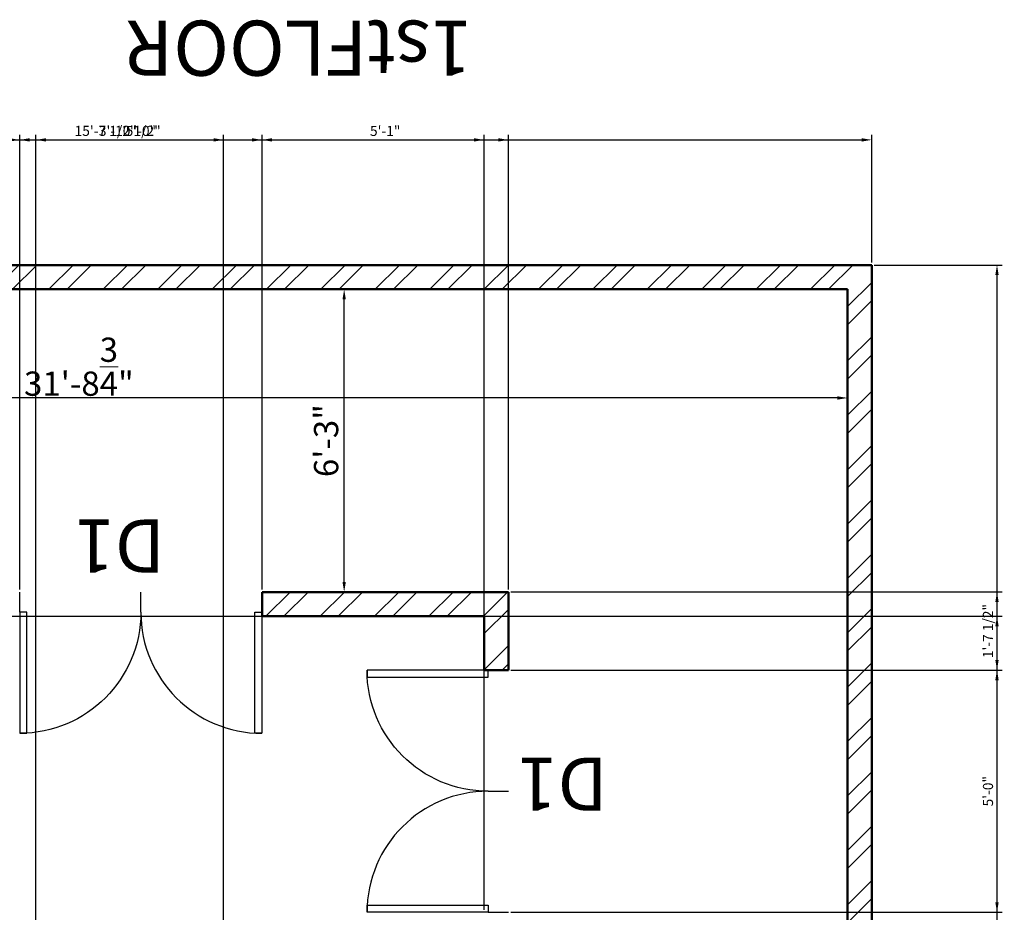
# Model space of a CAD drawing. Units: inches. Extents: x 244 to 2800, y 1060 to 1700.
# Tile 11 of 13: x 1781 to 2025, y 1473 to 1694. Entities that reach past the tile are written whole.
import ezdxf

# ---------------------------------------------------------------- set-up
doc = ezdxf.new("R2010")
doc.units = ezdxf.units.IN
for name, color, linetype, lineweight in [('A-ANNO-DIMS', 2, 'Continuous', 18), ('A-ANNO-TEXT', 1, 'Continuous', 18), ('A-DOOR', 5, 'Continuous', 25), ('A-WALL', 7, 'Continuous', 50), ('A-WALL-PATT', 8, 'Continuous', 13)]:
    doc.layers.add(name, color=color, linetype=linetype, lineweight=lineweight)
doc.styles.get("Standard").update_dxf_attribs({"font": 'arial.ttf'})
doc.dimstyles.new('ISO-25', dxfattribs={"dimtxt": 2.5, "dimasz": 2.5, "dimexe": 1.25, "dimexo": 0.625, "dimtad": 1, "dimlunit": 4, "dimtxsty": 'Standard', "dimcen": 2.5, "dimadec": 0, "dimazin": 0, "dimtfac": 1, "dimtmove": 0, "dimatfit": 3, "dimfxl": 1, "dimarcsym": 0})

# ---------------------------------------------------------------- blocks, each defined once
blk = doc.blocks.new('*U2')
for p, q in [((0, 0), (0, -5)), ((30, 0), (30, -5))]:
    blk.add_line(p, q)
blk.add_lwpolyline([(0, 0), (0, 30), (1.75, 30), (1.75, 0)], close=True)
blk.add_arc((0, 0), 30, 0, 90)
blk = doc.blocks.new('*D28')
at = {"layer": 'A-ANNO-DIMS', "color": 0, "lineweight": -2, "transparency": 16777216}
for p, q in [((1871.27, 1626.99), (1860.49, 1626.99)), ((1861.74, 1554.49), (1861.74, 1624.49)), ((1871.27, 1551.99), (1860.49, 1551.99))]:
    blk.add_line(p, q, dxfattribs=at)
at = {"layer": 'A-ANNO-DIMS', "color": 0, "transparency": 16777216}
for points in [[(1861.33, 1624.49), (1862.16, 1624.49), (1861.74, 1626.99)], [(1861.33, 1554.49), (1862.16, 1554.49), (1861.74, 1551.99)]]:
    blk.add_solid(points, dxfattribs=at)
at = {"layer": 'Defpoints', "color": 0, "transparency": 16777216}
for p in [(1861.74, 1626.99), (1871.9, 1626.99), (1871.9, 1551.99)]:
    blk.add_point(p, dxfattribs=at)
at = {"layer": 'A-ANNO-DIMS', "color": 0, "transparency": 16777216, "insert": (1858.05, 1589.49), "char_height": 6, "attachment_point": 5, "rotation": 90}
blk.add_mtext('6\'-3"', dxfattribs=at)
blk = doc.blocks.new('*D29')
at = {"layer": 'A-ANNO-DIMS', "color": 0, "lineweight": -2, "transparency": 16777216}
for p, q in [((1605.7, 1600.68), (1605.7, 1601.31)), ((1983.9, 1600.06), (1608.2, 1600.06)), ((1986.4, 1600.68), (1986.4, 1601.31))]:
    blk.add_line(p, q, dxfattribs=at)
at = {"layer": 'A-ANNO-DIMS', "color": 0, "transparency": 16777216}
for points in [[(1608.2, 1600.47), (1608.2, 1599.64), (1605.7, 1600.06)], [(1983.9, 1600.47), (1983.9, 1599.64), (1986.4, 1600.06)]]:
    blk.add_solid(points, dxfattribs=at)
at = {"layer": 'Defpoints', "color": 0, "transparency": 16777216}
for p in [(1605.7, 1600.06), (1605.7, 1600.06), (1986.4, 1600.06)]:
    blk.add_point(p, dxfattribs=at)
at = {"layer": 'A-ANNO-DIMS', "color": 0, "transparency": 16777216, "insert": (1796.05, 1607.8), "char_height": 6, "attachment_point": 5}
blk.add_mtext('31\'-8{\\H1x;\\S3/4;}"', dxfattribs=at)
blk = doc.blocks.new('*D74')
at = {"layer": 'A-ANNO-DIMS', "color": 0, "lineweight": -2, "transparency": 16777216}
for p, q in [((1512.4, 1633.61), (1512.4, 1665.24)), ((1992.4, 1633.61), (1992.4, 1665.24)), ((1514.9, 1663.99), (1989.9, 1663.99))]:
    blk.add_line(p, q, dxfattribs=at)
at = {"layer": 'A-ANNO-DIMS', "color": 0, "transparency": 16777216}
for points in [[(1514.9, 1664.4), (1514.9, 1663.57), (1512.4, 1663.99)], [(1989.9, 1664.4), (1989.9, 1663.57), (1992.4, 1663.99)]]:
    blk.add_solid(points, dxfattribs=at)
at = {"layer": 'Defpoints', "color": 0, "transparency": 16777216}
for p in [(1992.4, 1663.99), (1512.4, 1632.99), (1992.4, 1632.99)]:
    blk.add_point(p, dxfattribs=at)
at = {"layer": 'A-ANNO-DIMS', "color": 0, "transparency": 16777216, "insert": (1752.4, 1665.89), "char_height": 2.5, "attachment_point": 5}
blk.add_mtext('40\'-0"', dxfattribs=at)
blk = doc.blocks.new('*D75')
at = {"layer": 'A-ANNO-DIMS', "color": 0, "lineweight": -2, "transparency": 16777216}
for p, q in [((1993.02, 1632.99), (2024.65, 1632.99)), ((2023.4, 1095.49), (2023.4, 1630.49)), ((1993.02, 1092.99), (2024.65, 1092.99))]:
    blk.add_line(p, q, dxfattribs=at)
at = {"layer": 'A-ANNO-DIMS', "color": 0, "transparency": 16777216}
for points in [[(2022.98, 1630.49), (2023.81, 1630.49), (2023.4, 1632.99)], [(2022.98, 1095.49), (2023.81, 1095.49), (2023.4, 1092.99)]]:
    blk.add_solid(points, dxfattribs=at)
at = {"layer": 'Defpoints', "color": 0, "transparency": 16777216}
for p in [(1992.4, 1632.99), (2023.4, 1632.99), (1992.4, 1092.99)]:
    blk.add_point(p, dxfattribs=at)
at = {"layer": 'A-ANNO-DIMS', "color": 0, "transparency": 16777216, "insert": (2021.49, 1362.99), "char_height": 2.5, "attachment_point": 5, "rotation": 90}
blk.add_mtext('45\'-0"', dxfattribs=at)
blk = doc.blocks.new('*D78')
at = {"layer": 'A-ANNO-DIMS', "color": 0, "lineweight": -2, "transparency": 16777216}
for p, q in [((1756.81, 1552.61), (1756.81, 1665.24)), ((1781.4, 1552.61), (1781.4, 1665.24)), ((1759.31, 1663.99), (1778.9, 1663.99))]:
    blk.add_line(p, q, dxfattribs=at)
at = {"layer": 'A-ANNO-DIMS', "color": 0, "transparency": 16777216}
for points in [[(1759.31, 1664.4), (1759.31, 1663.57), (1756.81, 1663.99)], [(1778.9, 1664.4), (1778.9, 1663.57), (1781.4, 1663.99)]]:
    blk.add_solid(points, dxfattribs=at)
at = {"layer": 'Defpoints', "color": 0, "transparency": 16777216}
for p in [(1781.4, 1663.99), (1756.81, 1551.99), (1781.4, 1551.99)]:
    blk.add_point(p, dxfattribs=at)
at = {"layer": 'A-ANNO-DIMS', "color": 0, "transparency": 16777216, "insert": (1769.1, 1665.9), "char_height": 2.5, "attachment_point": 5}
blk.add_mtext('2\'-0 1/2"', dxfattribs=at)
blk = doc.blocks.new('*D79')
at = {"layer": 'A-ANNO-DIMS', "color": 0, "lineweight": -2, "transparency": 16777216}
for p, q in [((1781.4, 1552.61), (1781.4, 1665.24)), ((1841.4, 1552.61), (1841.4, 1665.24)), ((1783.9, 1663.99), (1838.9, 1663.99))]:
    blk.add_line(p, q, dxfattribs=at)
at = {"layer": 'A-ANNO-DIMS', "color": 0, "transparency": 16777216}
for points in [[(1783.9, 1664.4), (1783.9, 1663.57), (1781.4, 1663.99)], [(1838.9, 1664.4), (1838.9, 1663.57), (1841.4, 1663.99)]]:
    blk.add_solid(points, dxfattribs=at)
at = {"layer": 'Defpoints', "color": 0, "transparency": 16777216}
for p in [(1841.4, 1663.99), (1781.4, 1551.99), (1841.4, 1551.99)]:
    blk.add_point(p, dxfattribs=at)
at = {"layer": 'A-ANNO-DIMS', "color": 0, "transparency": 16777216, "insert": (1811.4, 1665.89), "char_height": 2.5, "attachment_point": 5}
blk.add_mtext('5\'-0"', dxfattribs=at)
blk = doc.blocks.new('*D80')
at = {"layer": 'A-ANNO-DIMS', "color": 0, "lineweight": -2, "transparency": 16777216}
for p, q in [((1841.4, 1552.61), (1841.4, 1665.24)), ((1902.4, 1552.61), (1902.4, 1665.24)), ((1843.9, 1663.99), (1899.9, 1663.99))]:
    blk.add_line(p, q, dxfattribs=at)
at = {"layer": 'A-ANNO-DIMS', "color": 0, "transparency": 16777216}
for points in [[(1843.9, 1664.4), (1843.9, 1663.57), (1841.4, 1663.99)], [(1899.9, 1664.4), (1899.9, 1663.57), (1902.4, 1663.99)]]:
    blk.add_solid(points, dxfattribs=at)
at = {"layer": 'Defpoints', "color": 0, "transparency": 16777216}
for p in [(1902.4, 1663.99), (1841.4, 1551.99), (1902.4, 1551.99)]:
    blk.add_point(p, dxfattribs=at)
at = {"layer": 'A-ANNO-DIMS', "color": 0, "transparency": 16777216, "insert": (1871.9, 1665.89), "char_height": 2.5, "attachment_point": 5}
blk.add_mtext('5\'-1"', dxfattribs=at)
blk = doc.blocks.new('*D87')
at = {"layer": 'A-ANNO-DIMS', "color": 0, "lineweight": -2, "transparency": 16777216}
for p, q in [((1537.02, 1545.99), (2024.65, 1545.99)), ((2023.4, 1375.49), (2023.4, 1543.49)), ((1537.02, 1372.99), (2024.65, 1372.99))]:
    blk.add_line(p, q, dxfattribs=at)
at = {"layer": 'A-ANNO-DIMS', "color": 0, "transparency": 16777216}
for points in [[(2022.98, 1543.49), (2023.81, 1543.49), (2023.4, 1545.99)], [(2022.98, 1375.49), (2023.81, 1375.49), (2023.4, 1372.99)]]:
    blk.add_solid(points, dxfattribs=at)
at = {"layer": 'Defpoints', "color": 0, "transparency": 16777216}
for p in [(1536.4, 1545.99), (2023.4, 1545.99), (1536.4, 1372.99)]:
    blk.add_point(p, dxfattribs=at)
at = {"layer": 'A-ANNO-DIMS', "color": 0, "transparency": 16777216, "insert": (2021.49, 1459.49), "char_height": 2.5, "attachment_point": 5, "rotation": 90}
blk.add_mtext('14\'-5"', dxfattribs=at)
blk = doc.blocks.new('*D90')
at = {"layer": 'A-ANNO-DIMS', "color": 0, "lineweight": -2, "transparency": 16777216}
for p, q in [((1708.9, 1491.26), (1708.9, 1665.24)), ((1896.4, 1473.26), (1896.4, 1665.24)), ((1711.4, 1663.99), (1893.9, 1663.99))]:
    blk.add_line(p, q, dxfattribs=at)
at = {"layer": 'A-ANNO-DIMS', "color": 0, "transparency": 16777216}
for points in [[(1711.4, 1664.4), (1711.4, 1663.57), (1708.9, 1663.99)], [(1893.9, 1664.4), (1893.9, 1663.57), (1896.4, 1663.99)]]:
    blk.add_solid(points, dxfattribs=at)
at = {"layer": 'Defpoints', "color": 0, "transparency": 16777216}
for p in [(1896.4, 1663.99), (1708.9, 1490.64), (1896.4, 1472.64)]:
    blk.add_point(p, dxfattribs=at)
at = {"layer": 'A-ANNO-DIMS', "color": 0, "transparency": 16777216, "insert": (1802.65, 1665.9), "char_height": 2.5, "attachment_point": 5}
blk.add_mtext('15\'-7 1/2"', dxfattribs=at)
blk = doc.blocks.new('*D100')
at = {"layer": 'A-ANNO-DIMS', "color": 0, "lineweight": -2, "transparency": 16777216}
for p, q in [((1903.02, 1532.64), (2024.65, 1532.64)), ((2023.4, 1475.14), (2023.4, 1530.14)), ((1903.02, 1472.64), (2024.65, 1472.64))]:
    blk.add_line(p, q, dxfattribs=at)
at = {"layer": 'A-ANNO-DIMS', "color": 0, "transparency": 16777216}
for points in [[(2022.98, 1530.14), (2023.81, 1530.14), (2023.4, 1532.64)], [(2022.98, 1475.14), (2023.81, 1475.14), (2023.4, 1472.64)]]:
    blk.add_solid(points, dxfattribs=at)
at = {"layer": 'Defpoints', "color": 0, "transparency": 16777216}
for p in [(1902.4, 1532.64), (2023.4, 1532.64), (1902.4, 1472.64)]:
    blk.add_point(p, dxfattribs=at)
at = {"layer": 'A-ANNO-DIMS', "color": 0, "transparency": 16777216, "insert": (2021.49, 1502.64), "char_height": 2.5, "attachment_point": 5, "rotation": 90}
blk.add_mtext('5\'-0"', dxfattribs=at)
blk = doc.blocks.new('*D101')
at = {"layer": 'A-ANNO-DIMS', "color": 0, "lineweight": -2, "transparency": 16777216}
for p, q in [((1903.02, 1551.99), (2024.65, 1551.99)), ((2023.4, 1535.14), (2023.4, 1549.49)), ((1903.02, 1532.64), (2024.65, 1532.64))]:
    blk.add_line(p, q, dxfattribs=at)
at = {"layer": 'A-ANNO-DIMS', "color": 0, "transparency": 16777216}
for points in [[(2022.98, 1549.49), (2023.81, 1549.49), (2023.4, 1551.99)], [(2022.98, 1535.14), (2023.81, 1535.14), (2023.4, 1532.64)]]:
    blk.add_solid(points, dxfattribs=at)
at = {"layer": 'Defpoints', "color": 0, "transparency": 16777216}
for p in [(1902.4, 1551.99), (2023.4, 1551.99), (1902.4, 1532.64)]:
    blk.add_point(p, dxfattribs=at)
at = {"layer": 'A-ANNO-DIMS', "color": 0, "transparency": 16777216, "insert": (2021.48, 1542.31), "char_height": 2.5, "attachment_point": 5, "rotation": 90}
blk.add_mtext('1\'-7 1/2"', dxfattribs=at)
blk = doc.blocks.new('*D104')
at = {"layer": 'A-ANNO-DIMS', "color": 0, "lineweight": -2, "transparency": 16777216}
for p, q in [((1785.4, 1201.61), (1785.4, 1665.24)), ((1831.9, 1206.11), (1831.9, 1665.24)), ((1787.9, 1663.99), (1829.4, 1663.99))]:
    blk.add_line(p, q, dxfattribs=at)
at = {"layer": 'A-ANNO-DIMS', "color": 0, "transparency": 16777216}
for points in [[(1787.9, 1664.4), (1787.9, 1663.57), (1785.4, 1663.99)], [(1829.4, 1664.4), (1829.4, 1663.57), (1831.9, 1663.99)]]:
    blk.add_solid(points, dxfattribs=at)
at = {"layer": 'Defpoints', "color": 0, "transparency": 16777216}
for p in [(1831.9, 1663.99), (1831.9, 1205.49), (1785.4, 1200.99)]:
    blk.add_point(p, dxfattribs=at)
at = {"layer": 'A-ANNO-DIMS', "color": 0, "transparency": 16777216, "insert": (1808.65, 1665.9), "char_height": 2.5, "attachment_point": 5}
blk.add_mtext('3\'-10 1/2"', dxfattribs=at)

msp = doc.modelspace()

# ---------------------------------------------------------------- hatches: boundary and pattern name
at = {"layer": 'A-WALL-PATT'}
h = msp.add_hatch(dxfattribs=at)
h.set_pattern_fill('ANSI32', color=256)
h.paths.add_polyline_path([(1992.396, 1092.986), (1992.396, 1632.986), (1512.396, 1632.986), (1512.396, 1092.986)])
h.paths.add_polyline_path([(1518.396, 1098.986), (1518.396, 1626.986), (1986.396, 1626.986), (1986.396, 1098.986), (1902.396, 1098.986)], flags=16)
h.paths.add_polyline_path([(1795.896, 1110.986), (1530.396, 1110.986), (1530.396, 1551.986), (1521.7, 1551.986), (1521.7, 1623.986), (1605.7, 1623.986), (1605.7, 1551.986), (1781.396, 1551.986), (1781.396, 1545.986), (1708.896, 1545.986), (1708.896, 1532.64), (1704.396, 1532.64), (1704.396, 1545.986), (1536.396, 1545.986), (1536.396, 1372.986), (1671.396, 1372.986), (1671.396, 1368.486), (1621.896, 1368.486), (1621.896, 1296.486), (1704.396, 1296.486), (1704.396, 1368.486), (1701.396, 1368.486), (1701.396, 1372.986), (1704.396, 1372.986), (1704.396, 1490.64), (1708.896, 1490.64), (1708.896, 1288.986), (1704.396, 1288.986), (1704.396, 1291.986), (1569.396, 1291.986), (1569.396, 1296.486), (1618.896, 1296.486), (1618.896, 1368.486), (1536.396, 1368.486), (1536.396, 1296.486), (1539.396, 1296.486), (1539.396, 1291.986), (1536.396, 1291.986), (1536.396, 1116.986), (1704.396, 1116.986), (1704.396, 1246.986), (1708.896, 1246.986), (1708.896, 1116.986), (1744.896, 1116.986), (1744.896, 1260.986), (1780.896, 1260.986), (1785.396, 1260.986), (1785.396, 1205.486), (1831.896, 1205.486), (1831.896, 1217.486), (1836.396, 1217.486), (1836.396, 1205.486), (1896.396, 1205.486), (1896.396, 1265.486), (1836.396, 1265.486), (1836.396, 1253.486), (1831.896, 1253.486), (1831.896, 1269.986), (1896.396, 1269.986), (1896.396, 1472.64), (1902.396, 1472.64), (1902.396, 1242.986), (1938.396, 1242.986), (1938.396, 1134.986), (1950.396, 1134.986), (1950.396, 1242.986), (1986.396, 1242.986), (1986.396, 1134.986), (1902.396, 1134.986), (1902.396, 1110.986), (1831.896, 1110.986), (1831.896, 1116.986), (1896.396, 1116.986), (1896.396, 1200.986), (1785.396, 1200.986), (1785.396, 1116.986), (1795.896, 1116.986)], flags=0)
h.paths.add_polyline_path([(1780.896, 1116.986), (1744.896, 1116.986), (1744.896, 1260.986), (1780.896, 1260.986)], flags=0)
h.paths.add_polyline_path([(1863.351, 1110.986), (1863.351, 1116.986), (1887.296, 1116.986), (1887.296, 1110.986)], flags=0)
h.paths.add_polyline_path([(1863.851, 1114.186), (1886.796, 1114.186), (1886.796, 1113.786), (1863.851, 1113.786)], flags=0)
h.paths.add_polyline_path([(1896.396, 1174.102), (1896.396, 1198.047), (1902.396, 1198.047), (1902.396, 1174.102)], flags=0)
h.paths.add_polyline_path([(1902.396, 1174.602), (1899.196, 1174.602), (1899.196, 1197.547), (1902.396, 1197.547)], flags=0)
h.paths.add_polyline_path([(1692.519, 1110.986), (1656.574, 1110.986), (1656.574, 1116.986), (1692.519, 1116.986)], flags=0)
h.paths.add_polyline_path([(1819.776, 1376.187), (1819.776, 1410.382, -0.249194), (1838.546, 1410.382), (1838.546, 1376.187, -0.249194)], flags=0)
h.paths.add_polyline_path([(1536.396, 1250.972), (1530.396, 1250.972), (1530.396, 1286.917), (1536.396, 1286.917)], flags=0)
h.paths.add_polyline_path([(1896.396, 1405.581), (1896.396, 1453.526), (1902.396, 1453.526), (1902.396, 1405.581)], flags=0)
h.paths.add_polyline_path([(1536.396, 1322.935), (1530.396, 1322.935), (1530.396, 1346.88), (1536.396, 1346.88)], flags=0)
h.paths.add_polyline_path([(1533.196, 1323.435), (1533.196, 1346.38), (1533.596, 1346.38), (1533.596, 1323.435)], flags=0)
h.paths.add_polyline_path([(1896.396, 1545.986), (1841.396, 1545.986), (1841.396, 1551.986), (1902.396, 1551.986), (1902.396, 1532.64), (1896.396, 1532.64)], flags=0)
h.paths.add_polyline_path([(1756.808, 1545.986), (1732.863, 1545.986), (1732.863, 1551.986), (1756.808, 1551.986)], flags=0)
h.paths.add_polyline_path([(1756.308, 1548.786), (1733.363, 1548.786), (1733.363, 1551.986), (1756.308, 1551.986)], flags=0)
h.paths.add_polyline_path([(1673.743, 1545.986), (1637.798, 1545.986), (1637.798, 1551.986), (1673.743, 1551.986)], flags=0)
h.paths.add_polyline_path([(1536.396, 1503.969), (1530.396, 1503.969), (1530.396, 1539.914), (1536.396, 1539.914)], flags=0)
h.paths.add_polyline_path([(1896.341, 1192.868), (1881.737, 1192.868), (1881.737, 1181.273), (1896.341, 1181.273)], flags=8)
h.paths.add_polyline_path([(1882.893, 1112.542), (1868.29, 1112.542), (1868.29, 1100.947), (1882.893, 1100.947)], flags=8)
h.paths.add_polyline_path([(1531.898, 1340.208), (1517.295, 1340.208), (1517.295, 1328.613), (1531.898, 1328.613)], flags=24)
h.paths.add_polyline_path([(1662.207, 1564.332), (1647.603, 1564.332), (1647.603, 1552.737), (1662.207, 1552.737)], flags=8)
h.paths.add_polyline_path([(1750.605, 1565.018), (1736.001, 1565.018), (1736.001, 1553.424), (1750.605, 1553.424)], flags=8)
h.paths.add_polyline_path([(1919.351, 1440.326), (1904.748, 1440.326), (1904.748, 1428.731), (1919.351, 1428.731)], flags=8)
h.paths.add_polyline_path([(1827.662, 1149.994), (1797.512, 1149.994), (1797.512, 1122.813), (1827.662, 1122.813)], flags=8)
h.paths.add_polyline_path([(1826.683, 1247.85), (1796.533, 1247.85), (1796.533, 1220.668), (1826.683, 1220.668)], flags=8)
h.paths.add_polyline_path([(1713.043, 1285.137), (1682.893, 1285.137), (1682.893, 1257.956), (1713.043, 1257.956)], flags=8)
h.paths.add_polyline_path([(1567.301, 1310.129), (1537.151, 1310.129), (1537.151, 1282.948), (1567.301, 1282.948)], flags=8)
h.paths.add_polyline_path([(1699.655, 1386.046), (1669.505, 1386.046), (1669.505, 1358.865), (1699.655, 1358.865)], flags=8)
h.paths.add_polyline_path([(1716.254, 1527.375), (1686.103, 1527.375), (1686.103, 1500.194), (1716.254, 1500.194)], flags=8)
h.paths.add_polyline_path([(1822.088, 1577.207), (1791.938, 1577.207), (1791.938, 1550.026), (1822.088, 1550.026)], flags=8)
h.paths.add_polyline_path([(1931.716, 1518.23), (1901.565, 1518.23), (1901.565, 1491.049), (1931.716, 1491.049)], flags=8)
h.paths.add_polyline_path([(1636.272, 1573.477), (1636.272, 1615.869), (1613.819, 1615.869), (1613.819, 1573.477)], flags=8)
h.paths.add_polyline_path([(1968.141, 1266.003), (1911.144, 1266.003), (1911.144, 1252.05), (1968.141, 1252.05)], flags=8)
h.paths.add_polyline_path([(1783.26, 1275.202), (1745.711, 1275.202), (1745.711, 1261.249), (1783.26, 1261.249)], flags=8)
h.paths.add_polyline_path([(1753.522, 1456.095), (1753.522, 1338.024), (1798.876, 1338.024), (1798.876, 1456.095)], flags=8)
h.paths.add_polyline_path([(1884.04, 1192.467), (1803.345, 1192.467), (1803.345, 1149.693), (1884.04, 1149.693)], flags=8)
h.paths.add_polyline_path([(1863.426, 1264.753), (1863.426, 1209.557), (1892.661, 1209.557), (1892.661, 1264.753)], flags=8)
h.paths.add_polyline_path([(1594.411, 1361.178), (1536.688, 1361.178), (1536.688, 1330.387), (1594.411, 1330.387)], flags=8)
h.paths.add_polyline_path([(1695.984, 1342.402), (1638.262, 1342.402), (1638.262, 1311.611), (1695.984, 1311.611)], flags=8)
h.paths.add_polyline_path([(1654.435, 1540.65), (1537.752, 1540.65), (1537.752, 1489.721), (1654.435, 1489.721)], flags=8)
h.paths.add_polyline_path([(1658.864, 1271.272), (1542.182, 1271.272), (1542.182, 1220.343), (1658.864, 1220.343)], flags=8)
h = msp.add_hatch(dxfattribs=at)
h.set_pattern_fill('ANSI32', color=256)
h.paths.add_polyline_path([(1902.396, 1551.986), (1841.396, 1551.986), (1841.396, 1545.986), (1896.396, 1545.986), (1896.396, 1532.64), (1897.396, 1532.64), (1902.396, 1532.64)])

# ---------------------------------------------------------------- linework, layer by layer
at = {"layer": 'A-WALL'}
for p, q in [((1992.396, 1632.986), (1512.396, 1632.986)), ((1992.396, 1092.986), (1992.396, 1632.986)), ((1986.396, 1626.986), (1518.396, 1626.986)), ((1986.396, 1098.986), (1986.396, 1626.986)), ((1841.396, 1545.986), (1841.396, 1551.986)), ((1841.396, 1551.986), (1902.396, 1551.986)), ((1902.396, 1532.64), (1902.396, 1551.986)), ((1841.396, 1545.986), (1896.396, 1545.986)), ((1896.396, 1532.64), (1896.396, 1545.986)), ((1896.317, 1532.64), (1902.396, 1532.64))]:
    msp.add_line(p, q, dxfattribs=at)

# ---------------------------------------------------------------- block references
at = {"layer": 'A-DOOR', "yscale": 0.9999956819955501, "zscale": 0.9999956819955501}
for p, xscale, rotation in [((1781.396, 1546.986), -0.9999956819955501, 180), ((1841.395, 1546.986), 0.9999956819955501, 180), ((1897.396, 1532.64), -0.9999956819955501, 90), ((1897.396, 1472.64), 0.9999956819955501, 90)]:
    msp.add_blockref('*U2', p, dxfattribs=dict(at, xscale=xscale, rotation=rotation))

# ---------------------------------------------------------------- texts
at = {"layer": 'A-ANNO-TEXT', "attachment_point": 1, "rotation": 180}
for s, width, gutter_width, insert, char_height in [('1stFLOOR', 25.27039, 68.243, (1893.513, 1679.874), 13.6485), ('D1', 20.58737, 65.951, (1817.369, 1556.761), 13.1902), ('D1', 20.58737, 65.951, (1926.997, 1497.783), 13.1902)]:
    msp.add_mtext_dynamic_manual_height_columns(s, width=width, gutter_width=gutter_width, heights=[0], dxfattribs=dict(at, insert=insert, char_height=char_height))

# ---------------------------------------------------------------- dimensions: what is measured, and where the dimension line sits
at = {"layer": 'A-ANNO-DIMS'}
for base, p1, p2, override, picture, middle in [((1896.396, 1663.986), (1708.896, 1490.64), (1896.396, 1472.64), {"dimdec": 1, "dimlfac": 1, "dimrnd": 0, "dimzin": 1, "dimdsep": 46, "dimlunit": 4, "dimfrac": 2}, '*D90', (1802.646, 1665.904)), ((1781.396, 1663.986), (1756.808, 1551.986), (1781.396, 1551.986), {"dimdec": 1, "dimlfac": 1, "dimrnd": 0, "dimzin": 1, "dimdsep": 46, "dimlunit": 4, "dimfrac": 2}, '*D78', (1769.102, 1665.904)), ((1831.896, 1663.986), (1785.396, 1200.986), (1831.896, 1205.486), {"dimdec": 1, "dimlfac": 1, "dimrnd": 0, "dimzin": 1, "dimdsep": 46, "dimlunit": 4, "dimfrac": 2}, '*D104', (1808.646, 1665.905)), ((1992.396, 1663.986), (1512.396, 1632.986), (1992.396, 1632.986), {"dimdec": 1, "dimlfac": 1, "dimrnd": 0, "dimzin": 1, "dimdsep": 46, "dimlunit": 4, "dimfrac": 2}, '*D74', (1752.396, 1665.888)), ((1841.396, 1663.986), (1781.396, 1551.986), (1841.396, 1551.986), {"dimdec": 1, "dimlfac": 1, "dimrnd": 0, "dimzin": 1, "dimdsep": 46, "dimlunit": 4, "dimfrac": 2}, '*D79', (1811.396, 1665.888)), ((1902.396, 1663.986), (1841.396, 1551.986), (1902.396, 1551.986), {"dimdec": 1, "dimlfac": 1, "dimrnd": 0, "dimzin": 1, "dimdsep": 46, "dimlunit": 4, "dimfrac": 2}, '*D80', (1871.896, 1665.888)), ((1605.7, 1600.057), (1986.396, 1600.057), (1605.7, 1600.057), {"dimtxt": 6, "dimclrd": 0, "dimclre": 0, "dimclrt": 0}, '*D29', (1796.048, 1607.8))]:
    dim = msp.add_linear_dim(base=base, p1=p1, p2=p2, dimstyle='ISO-25', override=override, dxfattribs=at)
    dim.commit()
    dim.dimension.update_dxf_attribs({"geometry": picture, "text_midpoint": middle})
for base, p1, p2, override, picture, middle in [((2023.396, 1632.986), (1992.396, 1092.986), (1992.396, 1632.986), {"dimdec": 1, "dimlfac": 1, "dimrnd": 0, "dimzin": 1, "dimdsep": 46, "dimlunit": 4, "dimfrac": 2}, '*D75', (2021.494, 1362.986)), ((1861.743, 1626.986), (1871.896, 1551.986), (1871.896, 1626.986), {"dimtxt": 6, "dimclrd": 0, "dimclre": 0, "dimclrt": 0}, '*D28', (1858.052, 1589.486)), ((2023.396, 1551.986), (1902.396, 1532.64), (1902.396, 1551.986), {"dimdec": 1, "dimlfac": 1, "dimrnd": 0, "dimzin": 1, "dimdsep": 46, "dimlunit": 4, "dimfrac": 2}, '*D101', (2021.478, 1542.313)), ((2023.396, 1545.986), (1536.396, 1372.986), (1536.396, 1545.986), {"dimdec": 1, "dimlfac": 1, "dimrnd": 0, "dimzin": 1, "dimdsep": 46, "dimlunit": 4, "dimfrac": 2}, '*D87', (2021.494, 1459.486)), ((2023.396, 1532.64), (1902.396, 1472.64), (1902.396, 1532.64), {"dimdec": 1, "dimlfac": 1, "dimrnd": 0, "dimzin": 1, "dimdsep": 46, "dimlunit": 4, "dimfrac": 2}, '*D100', (2021.494, 1502.64))]:
    dim = msp.add_linear_dim(base=base, p1=p1, p2=p2, angle=90, dimstyle='ISO-25', override=override, dxfattribs=at)
    dim.commit()
    dim.dimension.update_dxf_attribs({"geometry": picture, "text_midpoint": middle})

doc.saveas('drawing.dxf')
